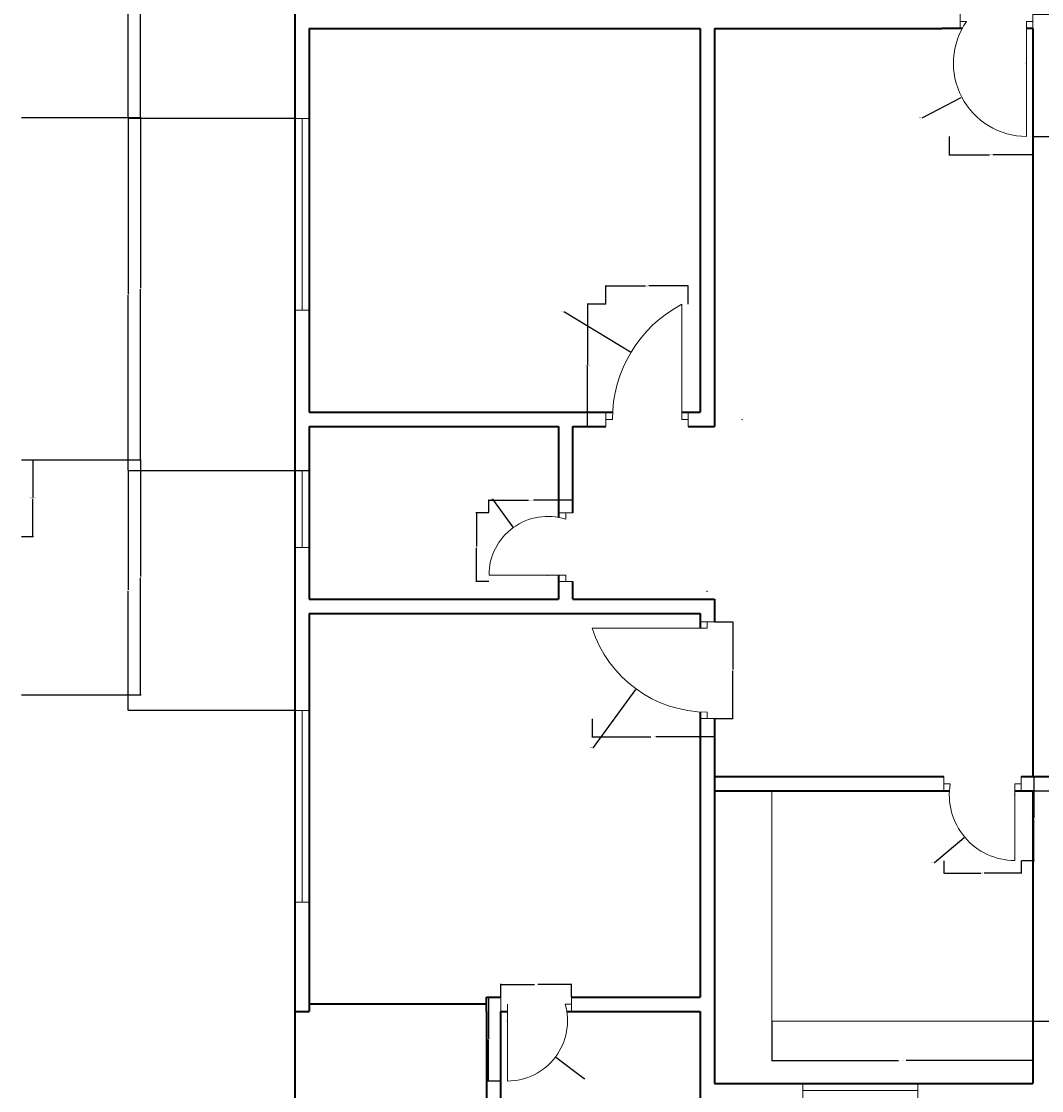
# Model space of a CAD drawing. Units: inches. Extents: x 992 to 2287, y 1476 to 2866.
# Tile 4 of 9: x 1531 to 1851, y 1652 to 1987. Entities that reach past the tile are written whole.
import ezdxf

# ---------------------------------------------------------------- set-up
doc = ezdxf.new("R2010")
doc.units = ezdxf.units.IN
for name, color, linetype, lineweight in [('A-ANNO-DIMS', 2, 'Continuous', 18), ('A-DOOR', 3, 'Continuous', 18), ('A-FLOR-CASE', 9, 'Continuous', 18), ('A-GLAZ', 4, 'Continuous', 18), ('A-WALL', 7, 'Continuous', 35)]:
    doc.layers.add(name, color=color, linetype=linetype, lineweight=lineweight)
doc.styles.get("Standard").update_dxf_attribs({"font": 'arial.ttf'})
doc.dimstyles.get("Standard").update_dxf_attribs({"dimtxt": 0.18, "dimasz": 0.18, "dimexe": 0.18, "dimexo": 0.0625, "dimgap": 0.09, "dimtad": 0, "dimtih": 1, "dimtoh": 1, "dimdec": 4, "dimzin": 0, "dimdsep": 46, "dimtxsty": 'Standard', "dimcen": 0.09, "dimadec": 0, "dimazin": 0, "dimtfac": 1, "dimtdec": 4, "dimtofl": 0, "dimtmove": 0, "dimatfit": 3, "dimfxl": 1, "dimtolj": 1, "dimtzin": 0, "dimarcsym": 0})

# ---------------------------------------------------------------- blocks, each defined once
blk = doc.blocks.new('DOOR-SINGLE-36IN-07')
for p, q in [((2.12, 38.25), (2.12, 33.75)), ((24.9, 33.75), (24.9, 38.25)), ((24.9, 38.25), (24.9, 36)), ((2.12, 36), (4.12, 36)), ((24.9, 36), (22.9, 36)), ((22.9, 36), (22.9, 0))]:
    blk.add_line(p, q)
blk.add_arc((22.9, 22.9), 22.9, 145.0915, 270)
blk = doc.blocks.new('DOOR-SINGLE-36IN-09')
for p, q in [((23.75, 2.25), (23.75, 38.25)), ((0, 4.5), (0, 0)), ((25.75, 4.5), (25.75, 0)), ((0, 0), (0, 2.25)), ((0, 2.25), (2, 2.25)), ((25.75, 2.25), (23.75, 2.25)), ((25.75, 0), (25.75, 2.25))]:
    blk.add_line(p, q)
blk.add_arc((42.67, 2.25), 40.67, 117.7196, 180)
blk = doc.blocks.new('DOOR-SINGLE-24IN-11')
for p, q in [((21.75, 21.48), (26.25, 21.48)), ((26.25, 21.48), (24, 21.48)), ((24, 21.48), (24, 19.48)), ((24, 2), (0, 2)), ((26.25, 0), (21.75, 0)), ((21.75, 0), (24, 0)), ((24, 0), (24, 2))]:
    blk.add_line(p, q)
blk.add_arc((18.36, 2), 18.36, 72.1205, 180)
blk = doc.blocks.new('DOOR-SINGLE-24IN-14')
for p, q in [((0, 21.75), (0, 26.25)), ((0, 26.25), (0, 24)), ((2, 24), (2, 0)), ((22.08, 24), (20.08, 24)), ((22.08, 26.25), (22.08, 21.75)), ((22.08, 21.75), (22.08, 24))]:
    blk.add_line(p, q)
blk.add_arc((2, 18.81), 18.81, 270, 16.0026)
blk = doc.blocks.new('DOOR-SINGLE-24IN-16')
for p, q in [((0, 26.25), (0, 21.75)), ((0, 21.75), (0, 24)), ((0, 24), (2, 24)), ((24.23, 24), (22.23, 24)), ((22.23, 24), (22.23, 0)), ((24.23, 21.75), (24.23, 26.25)), ((24.23, 26.25), (24.23, 24))]:
    blk.add_line(p, q)
blk.add_arc((22.23, 20.52), 20.52, 170.2522, 270)
blk = doc.blocks.new('DOOR-SINGLE-36IN-17')
for p, q in [((38.25, 30.21), (33.75, 30.21)), ((33.75, 30.21), (33.75, 30.21)), ((33.75, 30.21), (36, 30.21)), ((36, 30.21), (36, 28.21)), ((36, 28.21), (0, 28.21)), ((33.75, 0), (33.75, 0)), ((33.75, 0), (38.25, 0)), ((36, 0), (36, 2)), ((38.25, 0), (36, 0))]:
    blk.add_line(p, q)
blk.add_arc((36, 39.83), 37.83, 197.8869, 270)
blk = doc.blocks.new('WINDOW-60IN-A')
for p, q in [((4.5, 60), (0, 60)), ((0, 60), (2.25, 60)), ((2.25, 60), (2.25, 0)), ((2.25, 0), (0, 0)), ((0, 0), (4.5, 0))]:
    blk.add_line(p, q)
blk = doc.blocks.new('WINDOW-60IN-B')
for p, q in [((0, 4.5), (0, 0)), ((60, 2.25), (60, 4.5)), ((60, 4.5), (60, 0)), ((0, 0), (0, 2.25)), ((0, 2.25), (60, 2.25))]:
    blk.add_line(p, q)
blk = doc.blocks.new('WINDOW-36IN')
for p, q in [((0, 4.5), (0, 0)), ((36, 2.25), (36, 4.5)), ((36, 4.5), (36, 0)), ((0, 0), (0, 2.25)), ((0, 2.25), (36, 2.25))]:
    blk.add_line(p, q)
blk = doc.blocks.new('WINDOW-24IN-C')
for p, q in [((0, 24), (4.5, 24)), ((4.5, 24), (2.25, 24)), ((2.25, 24), (2.25, 0)), ((4.5, 0), (0, 0)), ((2.25, 0), (4.5, 0))]:
    blk.add_line(p, q)
blk = doc.blocks.new('COUNTER-L-SOUTHWEST')
for p, q in [((0, 72.06), (0, 0)), ((0, 0), (81.77, 0)), ((81.77, 0), (81.77, 0))]:
    blk.add_line(p, q)
blk = doc.blocks.new('*D45')
at = {"layer": 'A-ANNO-DIMS', "color": 0, "lineweight": -2, "transparency": 16777216}
for p, q in [((1531.36, 1849.65), (1535.07, 1849.65)), ((1534.89, 1849.47), (1534.89, 1837.83)), ((1534.89, 1825.83), (1534.89, 1837.47)), ((1531.36, 1825.65), (1535.07, 1825.65))]:
    blk.add_line(p, q, dxfattribs=at)
at = {"layer": 'A-ANNO-DIMS', "color": 0, "transparency": 16777216}
for points in [[(1534.86, 1849.47), (1534.92, 1849.47), (1534.89, 1849.65)], [(1534.86, 1825.83), (1534.92, 1825.83), (1534.89, 1825.65)]]:
    blk.add_solid(points, dxfattribs=at)
at = {"layer": 'Defpoints', "color": 0, "transparency": 16777216}
for p in [(1531.29, 1849.65), (1534.89, 1849.65), (1531.29, 1825.65)]:
    blk.add_point(p, dxfattribs=at)
at = {"layer": 'A-ANNO-DIMS', "color": 0, "transparency": 16777216, "insert": (1534.89, 1837.65), "char_height": 0.18, "attachment_point": 5}
blk.add_mtext('\\A1;WINDOW 24 TYP.', dxfattribs=at)
blk = doc.blocks.new('*D61')
at = {"layer": 'A-ANNO-DIMS', "color": 0, "lineweight": -2, "transparency": 16777216}
for p, q in [((1847.96, 1989.04), (1853.81, 1989.04)), ((1853.63, 1988.86), (1853.63, 1970.1)), ((1853.63, 1950.97), (1853.63, 1969.74)), ((1847.96, 1950.79), (1853.81, 1950.79))]:
    blk.add_line(p, q, dxfattribs=at)
at = {"layer": 'A-ANNO-DIMS', "color": 0, "transparency": 16777216}
for points in [[(1853.6, 1988.86), (1853.66, 1988.86), (1853.63, 1989.04)], [(1853.6, 1950.97), (1853.66, 1950.97), (1853.63, 1950.79)]]:
    blk.add_solid(points, dxfattribs=at)
at = {"layer": 'Defpoints', "color": 0, "transparency": 16777216}
for p in [(1847.89, 1989.04), (1853.63, 1989.04), (1847.89, 1950.79)]:
    blk.add_point(p, dxfattribs=at)
at = {"layer": 'A-ANNO-DIMS', "color": 0, "transparency": 16777216, "insert": (1853.63, 1969.92), "char_height": 0.18, "attachment_point": 5}
blk.add_mtext('\\A1;D07 38 TYP.', dxfattribs=at)
blk = doc.blocks.new('*D62')
at = {"layer": 'A-ANNO-DIMS', "color": 0, "lineweight": -2, "transparency": 16777216}
for p, q in [((1821.65, 1950.73), (1821.65, 1944.88)), ((1847.89, 1950.73), (1847.89, 1944.88)), ((1821.83, 1945.06), (1834.24, 1945.06)), ((1847.71, 1945.06), (1835.3, 1945.06))]:
    blk.add_line(p, q, dxfattribs=at)
at = {"layer": 'A-ANNO-DIMS', "color": 0, "transparency": 16777216}
for points in [[(1821.83, 1945.09), (1821.83, 1945.03), (1821.65, 1945.06)], [(1847.71, 1945.09), (1847.71, 1945.03), (1847.89, 1945.06)]]:
    blk.add_solid(points, dxfattribs=at)
at = {"layer": 'Defpoints', "color": 0, "transparency": 16777216}
for p in [(1821.65, 1950.79), (1847.89, 1950.79), (1847.89, 1945.06)]:
    blk.add_point(p, dxfattribs=at)
at = {"layer": 'A-ANNO-DIMS', "color": 0, "transparency": 16777216, "insert": (1834.77, 1945.06), "char_height": 0.18, "attachment_point": 5}
blk.add_mtext('\\A1;26 TYP.', dxfattribs=at)
blk = doc.blocks.new('*D65')
at = {"layer": 'A-ANNO-DIMS', "color": 0, "lineweight": -2, "transparency": 16777216}
for p, q in [((1714.19, 1898.29), (1708.34, 1898.29)), ((1708.52, 1898.11), (1708.52, 1879.35)), ((1708.52, 1860.22), (1708.52, 1878.99)), ((1714.19, 1860.04), (1708.34, 1860.04))]:
    blk.add_line(p, q, dxfattribs=at)
at = {"layer": 'A-ANNO-DIMS', "color": 0, "transparency": 16777216}
for points in [[(1708.49, 1898.11), (1708.55, 1898.11), (1708.52, 1898.29)], [(1708.49, 1860.22), (1708.55, 1860.22), (1708.52, 1860.04)]]:
    blk.add_solid(points, dxfattribs=at)
at = {"layer": 'Defpoints', "color": 0, "transparency": 16777216}
for p in [(1708.52, 1898.29), (1714.25, 1898.29), (1714.25, 1860.04)]:
    blk.add_point(p, dxfattribs=at)
at = {"layer": 'A-ANNO-DIMS', "color": 0, "transparency": 16777216, "insert": (1708.52, 1879.17), "char_height": 0.18, "attachment_point": 5}
blk.add_mtext('\\A1;D09 38 TYP.', dxfattribs=at)
blk = doc.blocks.new('*D66')
at = {"layer": 'A-ANNO-DIMS', "color": 0, "lineweight": -2, "transparency": 16777216}
for p, q in [((1714.25, 1898.36), (1714.25, 1904.21)), ((1714.43, 1904.03), (1726.6, 1904.03)), ((1739.82, 1904.03), (1727.66, 1904.03)), ((1740, 1898.36), (1740, 1904.21))]:
    blk.add_line(p, q, dxfattribs=at)
at = {"layer": 'A-ANNO-DIMS', "color": 0, "transparency": 16777216}
for points in [[(1714.43, 1904.06), (1714.43, 1904), (1714.25, 1904.03)], [(1739.82, 1904.06), (1739.82, 1904), (1740, 1904.03)]]:
    blk.add_solid(points, dxfattribs=at)
at = {"layer": 'Defpoints', "color": 0, "transparency": 16777216}
for p in [(1740, 1904.03), (1714.25, 1898.29), (1740, 1898.29)]:
    blk.add_point(p, dxfattribs=at)
at = {"layer": 'A-ANNO-DIMS', "color": 0, "transparency": 16777216, "insert": (1727.13, 1904.03), "char_height": 0.18, "attachment_point": 5}
blk.add_mtext('\\A1;26 TYP.', dxfattribs=at)
blk = doc.blocks.new('*D69')
at = {"layer": 'A-ANNO-DIMS', "color": 0, "lineweight": -2, "transparency": 16777216}
for p, q in [((1677.64, 1833.11), (1677.64, 1837.16)), ((1677.82, 1836.98), (1689.98, 1836.98)), ((1703.71, 1836.98), (1691.56, 1836.98)), ((1703.89, 1833.11), (1703.89, 1837.16))]:
    blk.add_line(p, q, dxfattribs=at)
at = {"layer": 'A-ANNO-DIMS', "color": 0, "transparency": 16777216}
for points in [[(1677.82, 1837.01), (1677.82, 1836.95), (1677.64, 1836.98)], [(1703.71, 1837.01), (1703.71, 1836.95), (1703.89, 1836.98)]]:
    blk.add_solid(points, dxfattribs=at)
at = {"layer": 'Defpoints', "color": 0, "transparency": 16777216}
for p in [(1703.89, 1836.98), (1677.64, 1833.04), (1703.89, 1833.04)]:
    blk.add_point(p, dxfattribs=at)
at = {"layer": 'A-ANNO-DIMS', "color": 0, "transparency": 16777216, "insert": (1690.77, 1836.98), "char_height": 0.18, "attachment_point": 5}
blk.add_mtext('\\A1;D11 26 TYP.', dxfattribs=at)
blk = doc.blocks.new('*D70')
at = {"layer": 'A-ANNO-DIMS', "color": 0, "lineweight": -2, "transparency": 16777216}
for p, q in [((1677.58, 1833.04), (1673.53, 1833.04)), ((1673.71, 1832.86), (1673.71, 1822.49)), ((1673.71, 1811.75), (1673.71, 1822.12)), ((1677.58, 1811.57), (1673.53, 1811.57))]:
    blk.add_line(p, q, dxfattribs=at)
at = {"layer": 'A-ANNO-DIMS', "color": 0, "transparency": 16777216}
for points in [[(1673.68, 1832.86), (1673.74, 1832.86), (1673.71, 1833.04)], [(1673.68, 1811.75), (1673.74, 1811.75), (1673.71, 1811.57)]]:
    blk.add_solid(points, dxfattribs=at)
at = {"layer": 'Defpoints', "color": 0, "transparency": 16777216}
for p in [(1673.71, 1833.04), (1677.64, 1833.04), (1677.64, 1811.57)]:
    blk.add_point(p, dxfattribs=at)
at = {"layer": 'A-ANNO-DIMS', "color": 0, "transparency": 16777216, "insert": (1673.71, 1822.3), "char_height": 0.18, "attachment_point": 5}
blk.add_mtext('\\A1;21 TYP.', dxfattribs=at)
blk = doc.blocks.new('*D75')
at = {"layer": 'A-ANNO-DIMS', "color": 0, "lineweight": -2, "transparency": 16777216}
for p, q in [((1681.33, 1681.54), (1677.28, 1681.54)), ((1677.46, 1681.36), (1677.46, 1668.6)), ((1677.46, 1655.47), (1677.46, 1668.24)), ((1681.33, 1655.29), (1677.28, 1655.29))]:
    blk.add_line(p, q, dxfattribs=at)
at = {"layer": 'A-ANNO-DIMS', "color": 0, "transparency": 16777216}
for points in [[(1677.43, 1681.36), (1677.49, 1681.36), (1677.46, 1681.54)], [(1677.43, 1655.47), (1677.49, 1655.47), (1677.46, 1655.29)]]:
    blk.add_solid(points, dxfattribs=at)
at = {"layer": 'Defpoints', "color": 0, "transparency": 16777216}
for p in [(1677.46, 1681.54), (1681.39, 1681.54), (1681.39, 1655.29)]:
    blk.add_point(p, dxfattribs=at)
at = {"layer": 'A-ANNO-DIMS', "color": 0, "transparency": 16777216, "insert": (1677.46, 1668.42), "char_height": 0.18, "attachment_point": 5}
blk.add_mtext('\\A1;D14 26 TYP.', dxfattribs=at)
blk = doc.blocks.new('*D76')
at = {"layer": 'A-ANNO-DIMS', "color": 0, "lineweight": -2, "transparency": 16777216}
for p, q in [((1681.39, 1681.61), (1681.39, 1685.66)), ((1681.57, 1685.48), (1691.91, 1685.48)), ((1703.3, 1685.48), (1692.97, 1685.48)), ((1703.48, 1681.61), (1703.48, 1685.66))]:
    blk.add_line(p, q, dxfattribs=at)
at = {"layer": 'A-ANNO-DIMS', "color": 0, "transparency": 16777216}
for points in [[(1681.57, 1685.51), (1681.57, 1685.45), (1681.39, 1685.48)], [(1703.3, 1685.51), (1703.3, 1685.45), (1703.48, 1685.48)]]:
    blk.add_solid(points, dxfattribs=at)
at = {"layer": 'Defpoints', "color": 0, "transparency": 16777216}
for p in [(1703.48, 1685.48), (1681.39, 1681.54), (1703.48, 1681.54)]:
    blk.add_point(p, dxfattribs=at)
at = {"layer": 'A-ANNO-DIMS', "color": 0, "transparency": 16777216, "insert": (1692.44, 1685.48), "char_height": 0.18, "attachment_point": 5}
blk.add_mtext('\\A1;22 TYP.', dxfattribs=at)
blk = doc.blocks.new('*D79')
at = {"layer": 'A-ANNO-DIMS', "color": 0, "lineweight": -2, "transparency": 16777216}
for p, q in [((1844.28, 1750.54), (1848.34, 1750.54)), ((1848.16, 1750.36), (1848.16, 1737.6)), ((1848.16, 1724.47), (1848.16, 1737.24)), ((1844.28, 1724.29), (1848.34, 1724.29))]:
    blk.add_line(p, q, dxfattribs=at)
at = {"layer": 'A-ANNO-DIMS', "color": 0, "transparency": 16777216}
for points in [[(1848.13, 1750.36), (1848.19, 1750.36), (1848.16, 1750.54)], [(1848.13, 1724.47), (1848.19, 1724.47), (1848.16, 1724.29)]]:
    blk.add_solid(points, dxfattribs=at)
at = {"layer": 'Defpoints', "color": 0, "transparency": 16777216}
for p in [(1844.22, 1750.54), (1848.16, 1750.54), (1844.22, 1724.29)]:
    blk.add_point(p, dxfattribs=at)
at = {"layer": 'A-ANNO-DIMS', "color": 0, "transparency": 16777216, "insert": (1848.16, 1737.42), "char_height": 0.18, "attachment_point": 5}
blk.add_mtext('\\A1;D16 26 TYP.', dxfattribs=at)
blk = doc.blocks.new('*D80')
at = {"layer": 'A-ANNO-DIMS', "color": 0, "lineweight": -2, "transparency": 16777216}
for p, q in [((1819.99, 1724.23), (1819.99, 1720.18)), ((1844.22, 1724.23), (1844.22, 1720.18)), ((1820.17, 1720.36), (1831.58, 1720.36)), ((1844.04, 1720.36), (1832.64, 1720.36))]:
    blk.add_line(p, q, dxfattribs=at)
at = {"layer": 'A-ANNO-DIMS', "color": 0, "transparency": 16777216}
for points in [[(1820.17, 1720.39), (1820.17, 1720.33), (1819.99, 1720.36)], [(1844.04, 1720.39), (1844.04, 1720.33), (1844.22, 1720.36)]]:
    blk.add_solid(points, dxfattribs=at)
at = {"layer": 'Defpoints', "color": 0, "transparency": 16777216}
for p in [(1819.99, 1724.29), (1844.22, 1724.29), (1844.22, 1720.36)]:
    blk.add_point(p, dxfattribs=at)
at = {"layer": 'A-ANNO-DIMS', "color": 0, "transparency": 16777216, "insert": (1832.11, 1720.36), "char_height": 0.18, "attachment_point": 5}
blk.add_mtext('\\A1;24 TYP.', dxfattribs=at)
blk = doc.blocks.new('*D81')
at = {"layer": 'A-ANNO-DIMS', "color": 0, "lineweight": -2, "transparency": 16777216}
for p, q in [((1709.93, 1768.65), (1709.93, 1762.79)), ((1748.18, 1768.65), (1748.18, 1762.79)), ((1710.11, 1762.97), (1728.27, 1762.97)), ((1748, 1762.97), (1729.85, 1762.97))]:
    blk.add_line(p, q, dxfattribs=at)
at = {"layer": 'A-ANNO-DIMS', "color": 0, "transparency": 16777216}
for points in [[(1710.11, 1763), (1710.11, 1762.94), (1709.93, 1762.97)], [(1748, 1763), (1748, 1762.94), (1748.18, 1762.97)]]:
    blk.add_solid(points, dxfattribs=at)
at = {"layer": 'Defpoints', "color": 0, "transparency": 16777216}
for p in [(1709.93, 1768.71), (1748.18, 1768.71), (1748.18, 1762.97)]:
    blk.add_point(p, dxfattribs=at)
at = {"layer": 'A-ANNO-DIMS', "color": 0, "transparency": 16777216, "insert": (1729.06, 1762.97), "char_height": 0.18, "attachment_point": 5}
blk.add_mtext('\\A1;D17 38 TYP.', dxfattribs=at)
blk = doc.blocks.new('*D82')
at = {"layer": 'A-ANNO-DIMS', "color": 0, "lineweight": -2, "transparency": 16777216}
for p, q in [((1748.25, 1798.92), (1754.1, 1798.92)), ((1753.92, 1798.74), (1753.92, 1784)), ((1753.92, 1768.89), (1753.92, 1783.64)), ((1748.25, 1768.71), (1754.1, 1768.71))]:
    blk.add_line(p, q, dxfattribs=at)
at = {"layer": 'A-ANNO-DIMS', "color": 0, "transparency": 16777216}
for points in [[(1753.89, 1798.74), (1753.95, 1798.74), (1753.92, 1798.92)], [(1753.89, 1768.89), (1753.95, 1768.89), (1753.92, 1768.71)]]:
    blk.add_solid(points, dxfattribs=at)
at = {"layer": 'Defpoints', "color": 0, "transparency": 16777216}
for p in [(1748.18, 1798.92), (1753.92, 1798.92), (1748.18, 1768.71)]:
    blk.add_point(p, dxfattribs=at)
at = {"layer": 'A-ANNO-DIMS', "color": 0, "transparency": 16777216, "insert": (1753.92, 1783.82), "char_height": 0.18, "attachment_point": 5}
blk.add_mtext('\\A1;30 TYP.', dxfattribs=at)
blk = doc.blocks.new('*D87')
at = {"layer": 'A-ANNO-DIMS', "color": 0, "lineweight": -2, "transparency": 16777216}
for p, q in [((1766.12, 1673.92), (1766.12, 1661.54)), ((1847.89, 1673.92), (1847.89, 1661.54)), ((1766.3, 1661.72), (1805.82, 1661.72)), ((1847.71, 1661.72), (1808.19, 1661.72))]:
    blk.add_line(p, q, dxfattribs=at)
at = {"layer": 'A-ANNO-DIMS', "color": 0, "transparency": 16777216}
for points in [[(1766.3, 1661.75), (1766.3, 1661.69), (1766.12, 1661.72)], [(1847.71, 1661.75), (1847.71, 1661.69), (1847.89, 1661.72)]]:
    blk.add_solid(points, dxfattribs=at)
at = {"layer": 'Defpoints', "color": 0, "transparency": 16777216}
for p in [(1766.12, 1673.98), (1847.89, 1673.98), (1847.89, 1661.72)]:
    blk.add_point(p, dxfattribs=at)
at = {"layer": 'A-ANNO-DIMS', "color": 0, "transparency": 16777216, "insert": (1807.01, 1661.72), "char_height": 0.18, "attachment_point": 5}
blk.add_mtext('\\A1;COUNTER 82 TYP.', dxfattribs=at)
blk = doc.blocks.new('*D88')
at = {"layer": 'A-ANNO-DIMS', "color": 0, "lineweight": -2, "transparency": 16777216}
for p, q in [((1847.96, 1746.04), (1860.34, 1746.04)), ((1860.16, 1745.86), (1860.16, 1710.19)), ((1860.16, 1674.16), (1860.16, 1709.83)), ((1847.96, 1673.98), (1860.34, 1673.98))]:
    blk.add_line(p, q, dxfattribs=at)
at = {"layer": 'A-ANNO-DIMS', "color": 0, "transparency": 16777216}
for points in [[(1860.13, 1745.86), (1860.19, 1745.86), (1860.16, 1746.04)], [(1860.13, 1674.16), (1860.19, 1674.16), (1860.16, 1673.98)]]:
    blk.add_solid(points, dxfattribs=at)
at = {"layer": 'Defpoints', "color": 0, "transparency": 16777216}
for p in [(1847.89, 1746.04), (1860.16, 1746.04), (1847.89, 1673.98)]:
    blk.add_point(p, dxfattribs=at)
at = {"layer": 'A-ANNO-DIMS', "color": 0, "transparency": 16777216, "insert": (1860.16, 1710.01), "char_height": 0.18, "attachment_point": 5}
blk.add_mtext('\\A1;72 TYP.', dxfattribs=at)
blk = doc.blocks.new('*D123')
at = {"layer": 'A-ANNO-DIMS', "color": 0, "lineweight": -2, "transparency": 16777216}
for p, q in [((1598.5, 2162.97), (1564.58, 2162.97)), ((1564.76, 2162.79), (1564.76, 2059.87)), ((1564.76, 1956.59), (1564.76, 2059.51)), ((1616.83, 1956.41), (1564.58, 1956.41))]:
    blk.add_line(p, q, dxfattribs=at)
at = {"layer": 'A-ANNO-DIMS', "color": 0, "transparency": 16777216}
for points in [[(1564.73, 2162.79), (1564.79, 2162.79), (1564.76, 2162.97)], [(1564.73, 1956.59), (1564.79, 1956.59), (1564.76, 1956.41)]]:
    blk.add_solid(points, dxfattribs=at)
at = {"layer": 'Defpoints', "color": 0, "transparency": 16777216}
for p in [(1564.76, 2162.97), (1598.56, 2162.97), (1616.89, 1956.41)]:
    blk.add_point(p, dxfattribs=at)
at = {"layer": 'A-ANNO-DIMS', "color": 0, "transparency": 16777216, "insert": (1564.76, 2059.69), "char_height": 0.18, "attachment_point": 5}
blk.add_mtext('\\A1;206.56', dxfattribs=at)
blk = doc.blocks.new('*D124')
at = {"layer": 'A-ANNO-DIMS', "color": 0, "lineweight": -2, "transparency": 16777216}
for p, q in [((1616.83, 1956.41), (1564.58, 1956.41)), ((1564.76, 1956.23), (1564.76, 1901.49)), ((1564.76, 1846.39), (1564.76, 1901.13)), ((1621.33, 1846.21), (1564.58, 1846.21))]:
    blk.add_line(p, q, dxfattribs=at)
at = {"layer": 'A-ANNO-DIMS', "color": 0, "transparency": 16777216}
for points in [[(1564.73, 1956.23), (1564.79, 1956.23), (1564.76, 1956.41)], [(1564.73, 1846.39), (1564.79, 1846.39), (1564.76, 1846.21)]]:
    blk.add_solid(points, dxfattribs=at)
at = {"layer": 'Defpoints', "color": 0, "transparency": 16777216}
for p in [(1564.76, 1956.41), (1616.89, 1956.41), (1621.39, 1846.21)]:
    blk.add_point(p, dxfattribs=at)
at = {"layer": 'A-ANNO-DIMS', "color": 0, "transparency": 16777216, "insert": (1564.76, 1901.31), "char_height": 0.18, "attachment_point": 5}
blk.add_mtext('\\A1;110.2', dxfattribs=at)
blk = doc.blocks.new('*D125')
at = {"layer": 'A-ANNO-DIMS', "color": 0, "lineweight": -2, "transparency": 16777216}
for p, q in [((1621.33, 1846.21), (1564.58, 1846.21)), ((1564.76, 1846.03), (1564.76, 1808.91)), ((1564.76, 1771.43), (1564.76, 1808.55)), ((1616.83, 1771.25), (1564.58, 1771.25))]:
    blk.add_line(p, q, dxfattribs=at)
at = {"layer": 'A-ANNO-DIMS', "color": 0, "transparency": 16777216}
for points in [[(1564.73, 1846.03), (1564.79, 1846.03), (1564.76, 1846.21)], [(1564.73, 1771.43), (1564.79, 1771.43), (1564.76, 1771.25)]]:
    blk.add_solid(points, dxfattribs=at)
at = {"layer": 'Defpoints', "color": 0, "transparency": 16777216}
for p in [(1564.76, 1846.21), (1621.39, 1846.21), (1616.89, 1771.25)]:
    blk.add_point(p, dxfattribs=at)
at = {"layer": 'A-ANNO-DIMS', "color": 0, "transparency": 16777216, "insert": (1564.76, 1808.73), "char_height": 0.18, "attachment_point": 5}
blk.add_mtext('\\A1;74.96', dxfattribs=at)
blk = doc.blocks.new('*D129')
at = {"layer": 'A-ANNO-DIMS', "color": 0, "lineweight": -2, "transparency": 16777216}
for p, q in [((1531.36, 2068.79), (1568.77, 2068.79)), ((1568.59, 2068.61), (1568.59, 2012.93)), ((1568.59, 1956.88), (1568.59, 2012.56)), ((1531.36, 1956.7), (1568.77, 1956.7))]:
    blk.add_line(p, q, dxfattribs=at)
at = {"layer": 'A-ANNO-DIMS', "color": 0, "transparency": 16777216}
for points in [[(1568.56, 2068.61), (1568.62, 2068.61), (1568.59, 2068.79)], [(1568.56, 1956.88), (1568.62, 1956.88), (1568.59, 1956.7)]]:
    blk.add_solid(points, dxfattribs=at)
at = {"layer": 'Defpoints', "color": 0, "transparency": 16777216}
for p in [(1531.29, 2068.79), (1568.59, 2068.79), (1531.29, 1956.7)]:
    blk.add_point(p, dxfattribs=at)
at = {"layer": 'A-ANNO-DIMS', "color": 0, "transparency": 16777216, "insert": (1568.59, 2012.74), "char_height": 0.18, "attachment_point": 5}
blk.add_mtext('\\A1;112.09', dxfattribs=at)
blk = doc.blocks.new('*D130')
at = {"layer": 'A-ANNO-DIMS', "color": 0, "lineweight": -2, "transparency": 16777216}
for p, q in [((1531.36, 1956.7), (1568.77, 1956.7)), ((1568.59, 1956.52), (1568.59, 1903.36)), ((1568.59, 1849.83), (1568.59, 1902.99)), ((1531.36, 1849.65), (1568.77, 1849.65))]:
    blk.add_line(p, q, dxfattribs=at)
at = {"layer": 'A-ANNO-DIMS', "color": 0, "transparency": 16777216}
for points in [[(1568.56, 1956.52), (1568.62, 1956.52), (1568.59, 1956.7)], [(1568.56, 1849.83), (1568.62, 1849.83), (1568.59, 1849.65)]]:
    blk.add_solid(points, dxfattribs=at)
at = {"layer": 'Defpoints', "color": 0, "transparency": 16777216}
for p in [(1531.29, 1956.7), (1568.59, 1956.7), (1531.29, 1849.65)]:
    blk.add_point(p, dxfattribs=at)
at = {"layer": 'A-ANNO-DIMS', "color": 0, "transparency": 16777216, "insert": (1568.59, 1903.17), "char_height": 0.18, "attachment_point": 5}
blk.add_mtext('\\A1;107.05', dxfattribs=at)
blk = doc.blocks.new('*D131')
at = {"layer": 'A-ANNO-DIMS', "color": 0, "lineweight": -2, "transparency": 16777216}
for p, q in [((1531.36, 1849.65), (1568.77, 1849.65)), ((1568.59, 1849.47), (1568.59, 1813.08)), ((1568.59, 1776.33), (1568.59, 1812.72)), ((1531.36, 1776.15), (1568.77, 1776.15))]:
    blk.add_line(p, q, dxfattribs=at)
at = {"layer": 'A-ANNO-DIMS', "color": 0, "transparency": 16777216}
for points in [[(1568.56, 1849.47), (1568.62, 1849.47), (1568.59, 1849.65)], [(1568.56, 1776.33), (1568.62, 1776.33), (1568.59, 1776.15)]]:
    blk.add_solid(points, dxfattribs=at)
at = {"layer": 'Defpoints', "color": 0, "transparency": 16777216}
for p in [(1531.29, 1849.65), (1568.59, 1849.65), (1531.29, 1776.15)]:
    blk.add_point(p, dxfattribs=at)
at = {"layer": 'A-ANNO-DIMS', "color": 0, "transparency": 16777216, "insert": (1568.59, 1812.9), "char_height": 0.18, "attachment_point": 5}
blk.add_mtext('\\A1;73.5', dxfattribs=at)
blk = doc.blocks.new('*D151')
at = {"layer": 'A-ANNO-DIMS', "color": 0, "lineweight": -2, "transparency": 16777216}
for p, q in [((1701.05, 1895.94), (1701.23, 1895.94)), ((1701.23, 1895.94), (1721.96, 1883.42)), ((1756.83, 1862.29), (1757.01, 1862.29)), ((1756.92, 1862.2), (1756.92, 1862.38))]:
    blk.add_line(p, q, dxfattribs=at)
at = {"layer": 'A-ANNO-DIMS', "color": 0, "transparency": 16777216}
blk.add_solid([(1721.97, 1883.44), (1721.94, 1883.39), (1722.11, 1883.32)], dxfattribs=at)
at = {"layer": 'Defpoints', "color": 0, "transparency": 16777216}
for p in [(1722.11, 1883.32), (1756.92, 1862.29)]:
    blk.add_point(p, dxfattribs=at)
at = {"layer": 'A-ANNO-DIMS', "color": 0, "transparency": 16777216, "insert": (1700.57, 1895.94), "char_height": 0.18, "attachment_point": 5}
blk.add_mtext('\\A1;R40.67', dxfattribs=at)
blk = doc.blocks.new('*D152')
at = {"layer": 'A-ANNO-DIMS', "color": 0, "lineweight": -2, "transparency": 16777216}
for p, q in [((1745.84, 1808.54), (1746.02, 1808.54)), ((1745.93, 1808.45), (1745.93, 1808.63)), ((1710.31, 1759.61), (1723.56, 1777.81)), ((1710.13, 1759.61), (1710.31, 1759.61))]:
    blk.add_line(p, q, dxfattribs=at)
at = {"layer": 'A-ANNO-DIMS', "color": 0, "transparency": 16777216}
blk.add_solid([(1723.54, 1777.83), (1723.59, 1777.8), (1723.67, 1777.96)], dxfattribs=at)
at = {"layer": 'Defpoints', "color": 0, "transparency": 16777216}
for p in [(1745.93, 1808.54), (1723.67, 1777.96)]:
    blk.add_point(p, dxfattribs=at)
at = {"layer": 'A-ANNO-DIMS', "color": 0, "transparency": 16777216, "insert": (1709.65, 1759.61), "char_height": 0.18, "attachment_point": 5}
blk.add_mtext('\\A1;R37.83', dxfattribs=at)
blk = doc.blocks.new('*D160')
at = {"layer": 'A-ANNO-DIMS', "color": 0, "lineweight": -2, "transparency": 16777216}
for p, q in [((1845.8, 1973.69), (1845.98, 1973.69)), ((1845.89, 1973.6), (1845.89, 1973.78)), ((1813.41, 1956.75), (1825.43, 1963.02)), ((1813.23, 1956.75), (1813.41, 1956.75))]:
    blk.add_line(p, q, dxfattribs=at)
at = {"layer": 'A-ANNO-DIMS', "color": 0, "transparency": 16777216}
blk.add_solid([(1825.42, 1963.04), (1825.45, 1962.99), (1825.59, 1963.1)], dxfattribs=at)
at = {"layer": 'Defpoints', "color": 0, "transparency": 16777216}
for p in [(1845.89, 1973.69), (1825.59, 1963.1)]:
    blk.add_point(p, dxfattribs=at)
at = {"layer": 'A-ANNO-DIMS', "color": 0, "transparency": 16777216, "insert": (1812.68, 1956.75), "char_height": 0.18, "attachment_point": 5}
blk.add_mtext('\\A1;R22.897', dxfattribs=at)
blk = doc.blocks.new('*D161')
at = {"layer": 'A-ANNO-DIMS', "color": 0, "lineweight": -2, "transparency": 16777216}
for p, q in [((1842.13, 1744.82), (1842.31, 1744.82)), ((1842.22, 1744.73), (1842.22, 1744.91)), ((1817.11, 1723.65), (1826.39, 1731.47)), ((1816.93, 1723.65), (1817.11, 1723.65))]:
    blk.add_line(p, q, dxfattribs=at)
at = {"layer": 'A-ANNO-DIMS', "color": 0, "transparency": 16777216}
blk.add_solid([(1826.37, 1731.5), (1826.41, 1731.45), (1826.53, 1731.59)], dxfattribs=at)
at = {"layer": 'Defpoints', "color": 0, "transparency": 16777216}
for p in [(1842.22, 1744.82), (1826.53, 1731.59)]:
    blk.add_point(p, dxfattribs=at)
at = {"layer": 'A-ANNO-DIMS', "color": 0, "transparency": 16777216, "insert": (1816.38, 1723.65), "char_height": 0.18, "attachment_point": 5}
blk.add_mtext('\\A1;R20.525', dxfattribs=at)
blk = doc.blocks.new('*D164')
at = {"layer": 'A-ANNO-DIMS', "color": 0, "lineweight": -2, "transparency": 16777216}
for p, q in [((1683.3, 1674.11), (1683.48, 1674.11)), ((1683.39, 1674.02), (1683.39, 1674.2)), ((1707.43, 1655.99), (1698.56, 1662.68)), ((1707.61, 1655.99), (1707.43, 1655.99))]:
    blk.add_line(p, q, dxfattribs=at)
at = {"layer": 'A-ANNO-DIMS', "color": 0, "transparency": 16777216}
blk.add_solid([(1698.58, 1662.7), (1698.55, 1662.65), (1698.42, 1662.78)], dxfattribs=at)
at = {"layer": 'Defpoints', "color": 0, "transparency": 16777216}
for p in [(1683.39, 1674.11), (1698.42, 1662.78)]:
    blk.add_point(p, dxfattribs=at)
at = {"layer": 'A-ANNO-DIMS', "color": 0, "transparency": 16777216, "insert": (1708.16, 1655.99), "char_height": 0.18, "attachment_point": 5}
blk.add_mtext('\\A1;R18.813', dxfattribs=at)
blk = doc.blocks.new('*D166')
at = {"layer": 'A-ANNO-DIMS', "color": 0, "lineweight": -2, "transparency": 16777216}
for p, q in [((1678.53, 1837.32), (1678.71, 1837.32)), ((1678.71, 1837.32), (1685.09, 1828.56)), ((1695.92, 1813.57), (1696.1, 1813.57)), ((1696.01, 1813.48), (1696.01, 1813.66))]:
    blk.add_line(p, q, dxfattribs=at)
at = {"layer": 'A-ANNO-DIMS', "color": 0, "transparency": 16777216}
blk.add_solid([(1685.12, 1828.57), (1685.07, 1828.54), (1685.2, 1828.41)], dxfattribs=at)
at = {"layer": 'Defpoints', "color": 0, "transparency": 16777216}
for p in [(1685.2, 1828.41), (1696.01, 1813.57)]:
    blk.add_point(p, dxfattribs=at)
at = {"layer": 'A-ANNO-DIMS', "color": 0, "transparency": 16777216, "insert": (1677.98, 1837.32), "char_height": 0.18, "attachment_point": 5}
blk.add_mtext('\\A1;R18.362', dxfattribs=at)

msp = doc.modelspace()

# ---------------------------------------------------------------- linework, layer by layer
at = {"layer": 'A-WALL'}
for p, q in [((1616.8946, 2280.0428), (1616.8946, 1677.0428)), ((1621.3946, 1984.5428), (1743.6835, 1984.5428)), ((1621.3946, 1984.5428), (1621.3946, 1864.5428)), ((1743.6835, 1984.5428), (1743.6835, 1864.5428)), ((1748.1835, 1984.5428), (1819.3946, 1984.5428)), ((1748.1835, 1984.5428), (1748.1835, 1860.0428)), ((1825.7334, 1984.5428), (1819.3946, 1984.5428)), ((1847.8946, 1984.5428), (1845.8946, 1984.5428)), ((1847.8946, 1984.5428), (1847.8946, 1750.5428)), ((1621.3946, 1864.5428), (1716.3152, 1864.5428)), ((1738.004, 1864.5428), (1743.6835, 1864.5428)), ((1621.3946, 1860.0428), (1699.3946, 1860.0428)), ((1621.3946, 1860.0428), (1621.3946, 1806.0428)), ((1621.3946, 1860.0428), (1699.3946, 1860.0428)), ((1699.3946, 1860.0428), (1699.3946, 1831.6144)), ((1703.8946, 1860.0428), (1714.253, 1860.0428)), ((1703.8946, 1833.0428), (1703.8946, 1860.0428)), ((1740.004, 1860.0428), (1748.1835, 1860.0428)), ((1699.3946, 1813.5672), (1699.3946, 1806.0428)), ((1703.8946, 1806.0428), (1703.8946, 1811.5672)), ((1621.3946, 1806.0428), (1699.3946, 1806.0428)), ((1703.8946, 1806.0428), (1748.1835, 1806.0428)), ((1748.1835, 1806.0428), (1748.1835, 1798.922)), ((1621.3946, 1801.5428), (1743.6835, 1801.5428)), ((1621.3946, 1801.5428), (1621.3946, 1681.5428)), ((1743.6835, 1801.5428), (1743.6835, 1796.922)), ((1743.6835, 1770.7792), (1743.6835, 1681.5428)), ((1748.1835, 1768.7122), (1748.1835, 1654.5428)), ((1748.1835, 1750.5428), (1819.9915, 1750.5428)), ((1844.22, 1750.5428), (1855.598, 1750.5428)), ((1748.1835, 1746.0428), (1821.7317, 1746.0428)), ((1842.22, 1746.0428), (1847.8946, 1746.0428)), ((1847.8946, 1746.0428), (1847.8946, 1654.5428)), ((1621.3946, 1681.5428), (1621.3946, 1677.0428)), ((1676.8946, 1679.2928), (1621.3946, 1679.2928)), ((1676.8946, 1681.5428), (1681.3946, 1681.5428)), ((1676.8946, 1677.0428), (1676.8946, 1681.5428)), ((1703.479, 1681.5428), (1743.6835, 1681.5428)), ((1616.8946, 1677.0428), (1621.3946, 1677.0428)), ((1616.8946, 1677.0428), (1621.3946, 1677.0428)), ((1616.8946, 1677.0428), (1616.8946, 1630.5428)), ((1676.8946, 1677.0428), (1676.8946, 1630.5428)), ((1681.3946, 1677.0428), (1683.3946, 1677.0428)), ((1681.3946, 1635.0428), (1681.3946, 1677.0428)), ((1701.9775, 1677.0428), (1743.6835, 1677.0428)), ((1743.6835, 1677.0428), (1743.6835, 1635.0428)), ((1748.1835, 1654.5428), (1847.8946, 1654.5428))]:
    msp.add_line(p, q, dxfattribs=at)

# ---------------------------------------------------------------- block references
at = {"layer": 'A-DOOR'}
for name, p in [('DOOR-SINGLE-36IN-07', (1822.998, 1950.793)), ('DOOR-SINGLE-36IN-09', (1714.253, 1860.043)), ('DOOR-SINGLE-24IN-11', (1677.645, 1811.567)), ('DOOR-SINGLE-36IN-17', (1709.933, 1768.712)), ('DOOR-SINGLE-24IN-16', (1819.991, 1724.293)), ('DOOR-SINGLE-24IN-14', (1681.395, 1655.293))]:
    msp.add_blockref(name, p, dxfattribs=at)
at = {"layer": 'A-FLOR-CASE'}
msp.add_blockref('COUNTER-L-SOUTHWEST', (1766.12, 1673.984), dxfattribs=at)
at = {"layer": 'A-GLAZ'}
for name, p in [('WINDOW-60IN-A', (1616.895, 1896.4076)), ('WINDOW-36IN', (1775.904, 1650.043))]:
    msp.add_blockref(name, p, dxfattribs=at)
at = {"layer": 'A-GLAZ', "rotation": 180}
msp.add_blockref('WINDOW-24IN-C', (1621.3941, 1846.2116), dxfattribs=at)
at = {"layer": 'A-GLAZ', "extrusion": (0, 0, -1), "zscale": -1, "rotation": 90}
msp.add_blockref('WINDOW-60IN-B', (-1616.8948, 1711.2492), dxfattribs=at)

# ---------------------------------------------------------------- dimensions: what is measured, and where the dimension line sits
at = {"layer": 'A-ANNO-DIMS'}
for base, p1, p2, override, picture, middle in [((1564.761, 2162.9718), (1616.8946, 1956.4076), (1598.561, 2162.9718), {"dimdec": 2, "dimlfac": 1, "dimrnd": 0, "dimzin": 0, "dimdsep": 46, "dimlunit": 2}, '*D123', (1564.761, 2059.6897)), ((1568.5936, 2068.7863), (1531.2936, 1956.7011), (1531.2936, 2068.7863), {"dimdec": 2, "dimlfac": 1, "dimrnd": 0, "dimzin": 0, "dimdsep": 46, "dimlunit": 2}, '*D129', (1568.5936, 2012.7437)), ((1568.5936, 1956.7011), (1531.2936, 1849.6487), (1531.2936, 1956.7011), {"dimdec": 2, "dimlfac": 1, "dimrnd": 0, "dimzin": 0, "dimdsep": 46, "dimlunit": 2}, '*D130', (1568.5936, 1903.1749)), ((1564.761, 1956.4076), (1621.3946, 1846.2119), (1616.8946, 1956.4076), {"dimdec": 1, "dimlfac": 1, "dimrnd": 0, "dimzin": 0, "dimdsep": 46, "dimlunit": 2}, '*D124', (1564.761, 1901.3097)), ((1568.5936, 1849.6487), (1531.2936, 1776.1494), (1531.2936, 1849.6487), {"dimdec": 1, "dimlfac": 1, "dimrnd": 0, "dimzin": 0, "dimdsep": 46, "dimlunit": 2}, '*D131', (1568.5936, 1812.899)), ((1564.761, 1846.2119), (1616.8946, 1771.2494), (1621.3946, 1846.2119), {"dimdec": 2, "dimlfac": 1, "dimrnd": 0, "dimzin": 0, "dimdsep": 46, "dimlunit": 2}, '*D125', (1564.761, 1808.7307))]:
    dim = msp.add_linear_dim(base=base, p1=p1, p2=p2, angle=90, dimstyle='Standard', override=override, dxfattribs=at)
    dim.commit()
    dim.dimension.update_dxf_attribs({"geometry": picture, "text_midpoint": middle})
for base, p1, p2, text, picture, middle in [((1853.6321, 1989.0428), (1847.8946, 1950.7928), (1847.8946, 1989.0428), 'D07 <> TYP.', '*D61', (1853.6321, 1969.9178)), ((1708.5155, 1898.2928), (1714.253, 1860.0428), (1714.253, 1898.2928), 'D09 <> TYP.', '*D65', (1708.5155, 1879.1678)), ((1534.8936, 1849.6487), (1531.2936, 1825.6487), (1531.2936, 1849.6487), 'WINDOW <> TYP.', '*D45', (1534.8936, 1837.6487)), ((1673.7071, 1833.0428), (1677.6446, 1811.5672), (1677.6446, 1833.0428), '<> TYP.', '*D70', (1673.7071, 1822.305)), ((1753.921, 1798.922), (1748.1835, 1768.7122), (1748.1835, 1798.922), '<> TYP.', '*D82', (1753.921, 1783.8171)), ((1848.1575, 1750.5428), (1844.22, 1724.2928), (1844.22, 1750.5428), 'D16 <> TYP.', '*D79', (1848.1575, 1737.4178)), ((1860.1607, 1746.0428), (1847.8946, 1673.9844), (1847.8946, 1746.0428), '<> TYP.', '*D88', (1860.1607, 1710.0136)), ((1677.4571, 1681.5428), (1681.3946, 1655.2928), (1681.3946, 1681.5428), 'D14 <> TYP.', '*D75', (1677.4571, 1668.4178))]:
    dim = msp.add_linear_dim(base=base, p1=p1, p2=p2, angle=90, text=text, dimstyle='Standard', override={"dimdec": 0, "dimlfac": 1, "dimrnd": 0, "dimzin": 0, "dimdsep": 46, "dimlunit": 2}, dxfattribs=at)
    dim.commit()
    dim.dimension.update_dxf_attribs({"geometry": picture, "text_midpoint": middle})
for center, mpoint, override, picture, middle in [((1845.8946, 1973.6896), (1825.5932, 1963.1011), {"dimdec": 3, "dimlfac": 1, "dimrnd": 0, "dimzin": 0, "dimdsep": 46, "dimlunit": 2}, '*D160', (1812.6825, 1956.7479)), ((1756.9201, 1862.2928), (1722.1129, 1883.3231), {"dimdec": 2, "dimlfac": 1, "dimrnd": 0, "dimzin": 0, "dimdsep": 46, "dimlunit": 2}, '*D151', (1700.5687, 1895.9413)), ((1696.007, 1813.5672), (1685.1979, 1828.4111), {"dimdec": 3, "dimlfac": 1, "dimrnd": 0, "dimzin": 0, "dimdsep": 46, "dimlunit": 2}, '*D166', (1677.9836, 1837.3175)), ((1745.9335, 1808.5406), (1723.668, 1777.959), {"dimdec": 2, "dimlfac": 1, "dimrnd": 0, "dimzin": 0, "dimdsep": 46, "dimlunit": 2}, '*D152', (1709.6488, 1759.61)), ((1842.22, 1744.8177), (1826.526, 1731.59), {"dimdec": 3, "dimlfac": 1, "dimrnd": 0, "dimzin": 0, "dimdsep": 46, "dimlunit": 2}, '*D161', (1816.3792, 1723.6535)), ((1683.3946, 1674.1063), (1698.4198, 1662.7842), {"dimdec": 3, "dimlfac": 1, "dimrnd": 0, "dimzin": 0, "dimdsep": 46, "dimlunit": 2}, '*D164', (1708.1647, 1655.9909))]:
    dim = msp.add_radius_dim(center=center, mpoint=mpoint, dimstyle='Standard', override=override, dxfattribs=at)
    dim.commit()
    dim.dimension.update_dxf_attribs({"geometry": picture, "text_midpoint": middle, "dimtype": 164})
for base, p1, p2, text, picture, middle in [((1847.8946, 1945.0553), (1821.6477, 1950.7928), (1847.8946, 1950.7928), '<> TYP.', '*D62', (1834.7712, 1945.0553)), ((1740.004, 1904.0303), (1714.253, 1898.2928), (1740.004, 1898.2928), '<> TYP.', '*D66', (1727.1285, 1904.0303)), ((1703.8946, 1836.9803), (1677.6446, 1833.0428), (1703.8946, 1833.0428), 'D11 <> TYP.', '*D69', (1690.7696, 1836.9803)), ((1748.1835, 1762.9747), (1709.9335, 1768.7122), (1748.1835, 1768.7122), 'D17 <> TYP.', '*D81', (1729.0585, 1762.9747)), ((1844.22, 1720.3553), (1819.9915, 1724.2928), (1844.22, 1724.2928), '<> TYP.', '*D80', (1832.1057, 1720.3553)), ((1703.479, 1685.4803), (1681.3946, 1681.5428), (1703.479, 1681.5428), '<> TYP.', '*D76', (1692.4368, 1685.4803)), ((1847.8946, 1661.7182), (1766.1205, 1673.9844), (1847.8946, 1673.9844), 'COUNTER <> TYP.', '*D87', (1807.0075, 1661.7182))]:
    dim = msp.add_linear_dim(base=base, p1=p1, p2=p2, text=text, dimstyle='Standard', override={"dimdec": 0, "dimlfac": 1, "dimrnd": 0, "dimzin": 0, "dimdsep": 46, "dimlunit": 2}, dxfattribs=at)
    dim.commit()
    dim.dimension.update_dxf_attribs({"geometry": picture, "text_midpoint": middle})

doc.saveas('drawing.dxf')
